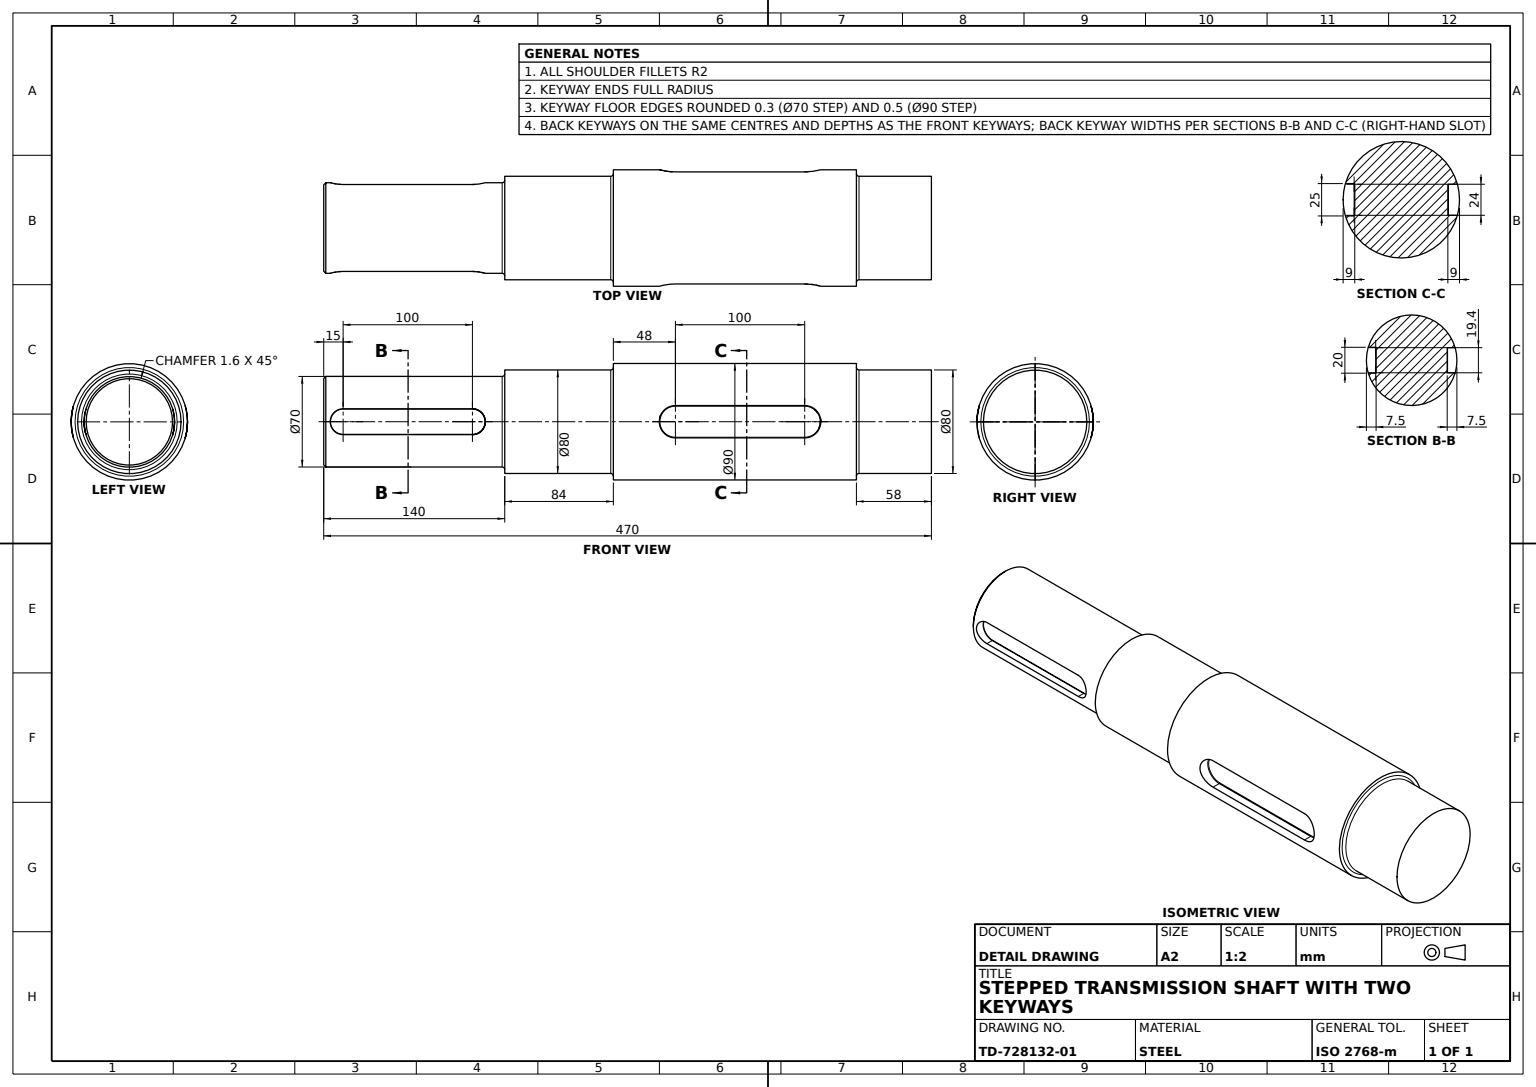
from build123d import *

# Parameters (mm, degrees)
END_CHAMFER_1_6X45DEG_SIZE        = 1.6
KEYWAY_A_CUT_7_5_DEEP_DEPTH       = 7.5
KEYWAY_A_EDGE_FILLET_R0_3_R       = 0.3
KEYWAY_B_CUT_9_DEEP_DEPTH         = 9
KEYWAY_B_EDGE_FILLET_R0_5_R       = 0.5
KEYWAY_B_SECOND_CUT_DEPTH         = 9
KEYWAY_A_SECOND_CUT_DEPTH         = 7.5
KEYWAY_B_SECOND_CUT_FILLET_R0_5_R = 0.5
KEYWAY_A_SECOND_CUT_FILLET_R0_3_R = 0.3
SHOULDER_FILLET_R2_R              = 2


with BuildPart() as part:
    # Shaft Profile Sketch → Stepped Shaft Body (revolve)
    with BuildSketch(Plane.XY, mode=Mode.PRIVATE) as stepped_shaft_body_sk:
        Polygon((0, 0), (0, 35), (140, 35), (140, 40), (224, 40), (224, 45), (412, 45), (412, 40), (470, 40), (470, 0), align=None)
    revolve(stepped_shaft_body_sk.sketch.rotate(Axis((0, 0, 0), (1, 0, 0)), 90), axis=Axis((0, 0, 0), (1, 0, 0)))

    # End Chamfer 1.6x45deg
    end_chamfer_1_6x45deg_edges = [part.edges().sort_by_distance(p)[0] for p in [
        (0, 0, -35),
    ]]
    chamfer(end_chamfer_1_6x45deg_edges, length=END_CHAMFER_1_6X45DEG_SIZE)

    # Keyway A Sketch → Keyway A Cut 7.5 Deep (cut)
    with BuildSketch(Plane.XY.offset(35)):
        with BuildLine():
            Line((15, 10), (115, 10))
            ThreePointArc((115, 10), (125, 0), (115, -10))
            Line((115, -10), (15, -10))
            ThreePointArc((15, -10), (5, 0), (15, 10))
        make_face()
    extrude(amount=-KEYWAY_A_CUT_7_5_DEEP_DEPTH, mode=Mode.SUBTRACT)

    # Keyway A Edge Fillet R0.3
    keyway_a_edge_fillet_r0_3_edges = [part.edges().sort_by_distance(p)[0] for p in [
        (5, 0, 27.5),
        (65, 10, 27.5),
        (125, 0, 27.5),
        (65, -10, 27.5),
    ]]
    fillet(keyway_a_edge_fillet_r0_3_edges, radius=KEYWAY_A_EDGE_FILLET_R0_3_R)

    # Keyway B Sketch → Keyway B Cut 9 Deep (cut)
    with BuildSketch(Plane.XY.offset(45)):
        with BuildLine():
            Line((272, 12.5), (372, 12.5))
            ThreePointArc((372, 12.5), (384.5, 0), (372, -12.5))
            Line((372, -12.5), (272, -12.5))
            ThreePointArc((272, -12.5), (259.5, 0), (272, 12.5))
        make_face()
    extrude(amount=-KEYWAY_B_CUT_9_DEEP_DEPTH, mode=Mode.SUBTRACT)

    # Keyway B Edge Fillet R0.5
    keyway_b_edge_fillet_r0_5_edges = [part.edges().sort_by_distance(p)[0] for p in [
        (259.5, 0, 36),
        (322, 12.5, 36),
        (384.5, 0, 36),
        (322, -12.5, 36),
    ]]
    fillet(keyway_b_edge_fillet_r0_5_edges, radius=KEYWAY_B_EDGE_FILLET_R0_5_R)

    # Keyway B Second Cut Sketch → Keyway B Second Cut (cut)
    with BuildSketch(Plane.XY.offset(-45)):
        with BuildLine():
            Line((372, 12), (272, 12))
            ThreePointArc((272, 12), (260, 0), (272, -12))
            Line((272, -12), (372, -12))
            ThreePointArc((372, -12), (384, 0), (372, 12))
        make_face()
    extrude(amount=KEYWAY_B_SECOND_CUT_DEPTH, mode=Mode.SUBTRACT)

    # Keyway A Second Cut Sketch → Keyway A Second Cut (cut)
    with BuildSketch(Plane.XY.offset(-35)):
        with BuildLine():
            Line((115, 9.7), (15, 9.7))
            ThreePointArc((15, 9.7), (5.3, 0), (15, -9.7))
            Line((15, -9.7), (115, -9.7))
            ThreePointArc((115, -9.7), (124.7, 0), (115, 9.7))
        make_face()
    extrude(amount=KEYWAY_A_SECOND_CUT_DEPTH, mode=Mode.SUBTRACT)

    # Keyway B Second Cut Fillet R0.5
    keyway_b_second_cut_fillet_r0_5_edges = [part.edges().sort_by_distance(p)[0] for p in [
        (384, 0, -36),
        (322, 12, -36),
        (260, 0, -36),
        (322, -12, -36),
    ]]
    fillet(keyway_b_second_cut_fillet_r0_5_edges, radius=KEYWAY_B_SECOND_CUT_FILLET_R0_5_R)

    # Keyway A Second Cut Fillet R0.3
    keyway_a_second_cut_fillet_r0_3_edges = [part.edges().sort_by_distance(p)[0] for p in [
        (124.7, 0, -27.5),
        (65, 9.7, -27.5),
        (5.3, 0, -27.5),
        (65, -9.7, -27.5),
    ]]
    fillet(keyway_a_second_cut_fillet_r0_3_edges, radius=KEYWAY_A_SECOND_CUT_FILLET_R0_3_R)

    # Shoulder Fillet R2
    shoulder_fillet_r2_edges = [part.edges().sort_by_distance(p)[0] for p in [
        (224, 0, -40),
        (140, 0, -35),
        (412, 0, -40),
    ]]
    fillet(shoulder_fillet_r2_edges, radius=SHOULDER_FILLET_R2_R)


solid = part.part
